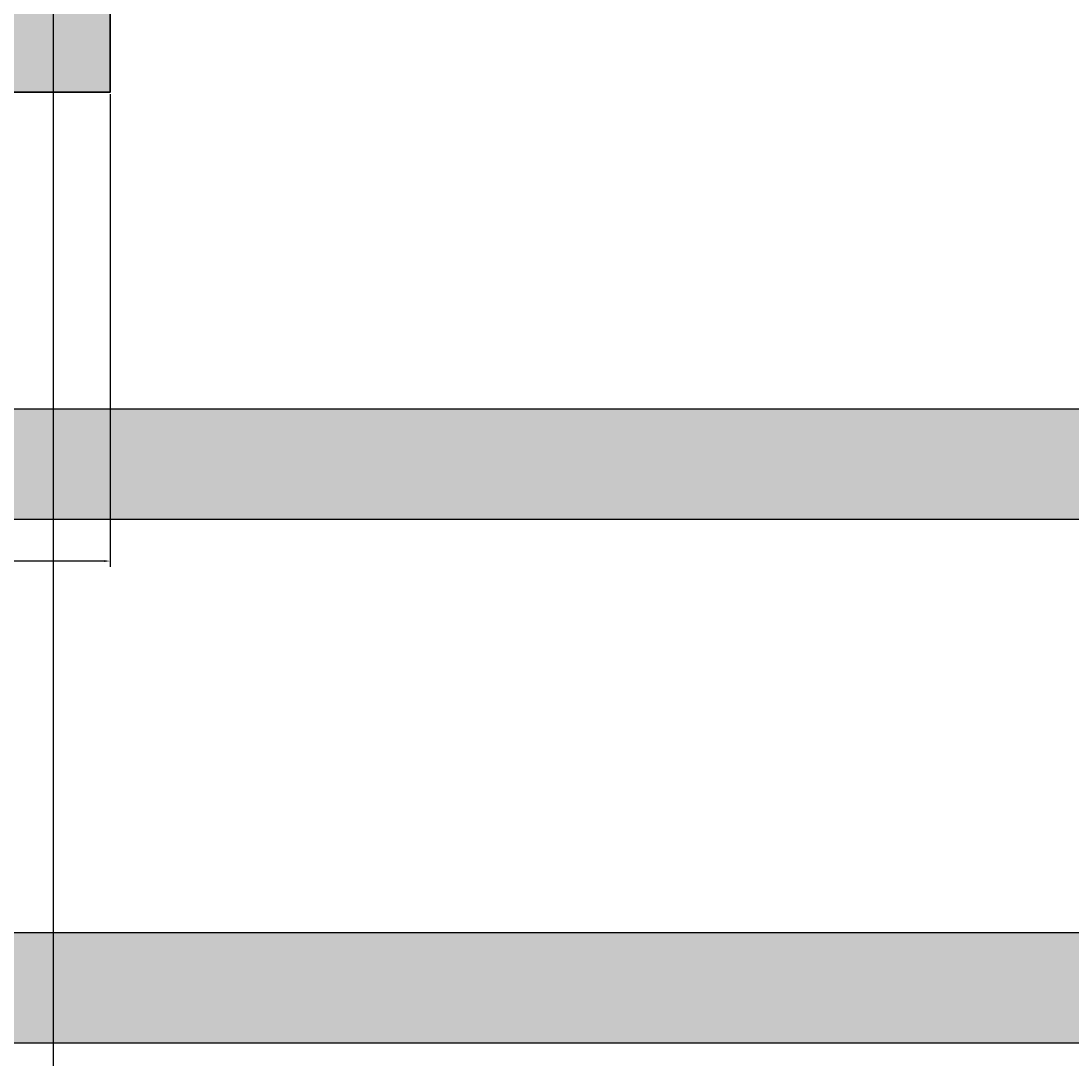
# Model space of a CAD drawing. Units: millimetres. Extents: x -11 to 280, y -4 to 208.
# Tile 4 of 55: x 28 to 61, y 54 to 87. Entities that reach past the tile are written whole.
import ezdxf

# ---------------------------------------------------------------- set-up
doc = ezdxf.new("R2010")
doc.units = ezdxf.units.MM
for name, color, linetype, lineweight in [('M-DIMS', 2, 'Continuous', 18), ('M-HYDR-EQPM', 7, 'Continuous', 35), ('M-HYDR-EQPM-PATT', 252, 'Continuous', 13), ('M-HYDR-RETN', 7, 'Continuous', 25)]:
    doc.layers.add(name, color=color, linetype=linetype, lineweight=lineweight)
doc.layers.add('M-HYDR-RETN-PATT', color=114, linetype='Continuous', lineweight=13, true_color=0x139b48)
doc.styles.get("Standard").update_dxf_attribs({"font": 'arial.ttf'})
doc.dimstyles.get("Standard").update_dxf_attribs({"dimtxt": 0.18, "dimasz": 0.18, "dimexe": 0.18, "dimexo": 0.0625, "dimgap": 0.09, "dimtad": 0, "dimtih": 1, "dimtoh": 1, "dimdec": 4, "dimzin": 0, "dimdsep": 46, "dimtxsty": 'Standard', "dimcen": 0.09, "dimadec": 0, "dimazin": 0, "dimtfac": 1, "dimtdec": 4, "dimtofl": 0, "dimtmove": 0, "dimatfit": 3, "dimfxl": 1, "dimtolj": 1, "dimtzin": 0, "dimarcsym": 0})

# ---------------------------------------------------------------- blocks, each defined once
blk = doc.blocks.new('*D4')
at = {"layer": 'Defpoints', "color": 0, "transparency": 16777216}
for p in [(4.763, 84.426), (266.035, 51.733), (266.035, -3.415)]:
    blk.add_point(p, dxfattribs=at)
at = {"layer": 'M-DIMS', "color": 0, "lineweight": -2, "transparency": 16777216}
for p, q in [((4.763, 84.364), (4.763, -3.595)), ((266.035, 51.67), (266.035, -3.595)), ((4.943, -3.415), (134.934, -3.415)), ((265.855, -3.415), (135.864, -3.415))]:
    blk.add_line(p, q, dxfattribs=at)
at = {"layer": 'M-DIMS', "color": 0, "transparency": 16777216}
for points in [[(4.943, -3.385), (4.943, -3.445), (4.763, -3.415)], [(265.855, -3.385), (265.855, -3.445), (266.035, -3.415)]]:
    blk.add_solid(points, dxfattribs=at)
at = {"layer": 'M-DIMS', "color": 0, "transparency": 16777216, "insert": (135.399, -3.415), "char_height": 0.18, "attachment_point": 5}
blk.add_mtext('\\A1;261.27', dxfattribs=at)
blk = doc.blocks.new('*D5')
at = {"layer": 'Defpoints', "color": 0, "transparency": 16777216}
for p in [(24.759, 192.645), (-10.087, 11.435), (261.686, 11.435)]:
    blk.add_point(p, dxfattribs=at)
at = {"layer": 'M-DIMS', "color": 0, "lineweight": -2, "transparency": 16777216}
for p, q in [((24.696, 192.645), (-10.267, 192.645)), ((-10.087, 192.465), (-10.087, 102.222)), ((-10.087, 11.615), (-10.087, 101.858)), ((261.624, 11.435), (-10.267, 11.435))]:
    blk.add_line(p, q, dxfattribs=at)
at = {"layer": 'M-DIMS', "color": 0, "transparency": 16777216}
for points in [[(-10.117, 192.465), (-10.057, 192.465), (-10.087, 192.645)], [(-10.117, 11.615), (-10.057, 11.615), (-10.087, 11.435)]]:
    blk.add_solid(points, dxfattribs=at)
at = {"layer": 'M-DIMS', "color": 0, "transparency": 16777216, "insert": (-10.087, 102.04), "char_height": 0.18, "attachment_point": 5}
blk.add_mtext('\\A1;181.2', dxfattribs=at)
blk = doc.blocks.new('*D23')
at = {"layer": 'Defpoints', "color": 0, "transparency": 16777216}
for p in [(29.201, 153.977), (66.388, 153.977), (66.388, -3.415)]:
    blk.add_point(p, dxfattribs=at)
at = {"layer": 'M-DIMS', "color": 0, "lineweight": -2, "transparency": 16777216}
for p, q in [((29.201, 153.914), (29.201, -3.595)), ((66.388, 153.914), (66.388, -3.595)), ((29.381, -3.415), (47.331, -3.415)), ((66.208, -3.415), (48.258, -3.415))]:
    blk.add_line(p, q, dxfattribs=at)
at = {"layer": 'M-DIMS', "color": 0, "transparency": 16777216}
for points in [[(29.381, -3.385), (29.381, -3.445), (29.201, -3.415)], [(66.208, -3.385), (66.208, -3.445), (66.388, -3.415)]]:
    blk.add_solid(points, dxfattribs=at)
at = {"layer": 'M-DIMS', "color": 0, "transparency": 16777216, "insert": (47.795, -3.415), "char_height": 0.18, "attachment_point": 5}
blk.add_mtext('\\A1;37.186', dxfattribs=at)
blk = doc.blocks.new('*D27')
at = {"layer": 'Defpoints', "color": 0, "transparency": 16777216}
for p in [(4.763, 84.426), (31.006, 84.426), (4.763, 69.576)]:
    blk.add_point(p, dxfattribs=at)
at = {"layer": 'M-DIMS', "color": 0, "lineweight": -2, "transparency": 16777216}
for p, q in [((4.763, 84.364), (4.763, 69.396)), ((31.006, 84.364), (31.006, 69.396)), ((4.943, 69.576), (17.49, 69.576)), ((30.826, 69.576), (18.28, 69.576))]:
    blk.add_line(p, q, dxfattribs=at)
at = {"layer": 'M-DIMS', "color": 0, "transparency": 16777216}
for points in [[(4.943, 69.606), (4.943, 69.546), (4.763, 69.576)], [(30.826, 69.606), (30.826, 69.546), (31.006, 69.576)]]:
    blk.add_solid(points, dxfattribs=at)
at = {"layer": 'M-DIMS', "color": 0, "transparency": 16777216, "insert": (17.885, 69.576), "char_height": 0.18, "attachment_point": 5}
blk.add_mtext('\\A1;26.24', dxfattribs=at)

msp = doc.modelspace()

# ---------------------------------------------------------------- hatches: boundary and pattern name
at = {"layer": 'M-HYDR-EQPM-PATT'}
h = msp.add_hatch(color=256, dxfattribs=at)
h.set_gradient(color1=(69, 84, 165), color2=(0, 0, 255), tint=1)
h.paths.add_polyline_path([(31.0059, 84.4261), (31.0059, 98.0213), (4.7635, 98.0213), (4.7635, 84.4261)])
at = {"layer": 'M-HYDR-RETN-PATT'}
h = msp.add_hatch(color=256, dxfattribs=at)
h.set_gradient(color1=(19, 155, 72), color2=(19, 155, 72), tint=1)
h.paths.add_polyline_path([(17.9701, 159.0814), (29.2015, 159.0814), (29.2015, 162.5814), (14.4701, 162.5814), (14.4701, 98.0213), (17.9701, 98.0213)])
h.paths.add_polyline_path([(17.9701, 84.4261), (14.4701, 84.4261), (14.4701, 54.3099), (156.2446, 54.3099), (156.2446, 57.8099), (17.9701, 57.8099)])
h.paths.add_polyline_path([(120.5137, 74.3991), (17.9701, 74.3991), (17.9701, 70.8991), (120.5137, 70.8991)], flags=17)
h.paths.add_polyline_path([(184.7092, 75.04, 0.4142136), (179.7092, 80.04), (156.2446, 80.04), (156.2446, 57.8099), (156.2446, 54.3099), (156.2446, 43.5991), (159.7446, 43.5991), (159.7446, 57.8099), (159.7446, 76.54), (176.2092, 76.54, -0.4142136), (181.2092, 71.54), (181.2092, 57.8099), (159.7446, 57.8099), (159.7446, 54.3099), (184.7092, 54.3099)])

# ---------------------------------------------------------------- linework, layer by layer
at = {"layer": 'M-HYDR-EQPM'}
msp.add_lwpolyline([(4.7635, 98.0213), (31.0059, 98.0213), (31.0059, 84.4261), (4.7635, 84.4261)], close=True, dxfattribs=at)
at = {"layer": 'M-HYDR-RETN'}
for points in [[(14.4701, 84.4261), (14.4701, 54.3099), (156.2446, 54.3099)], [(17.9701, 84.4261), (17.9701, 57.8099), (156.2446, 57.8099)], [(17.9701, 74.3991), (120.5137, 74.3991)], [(17.9701, 70.8991), (120.5137, 70.8991)]]:
    msp.add_lwpolyline(points, dxfattribs=at)

# ---------------------------------------------------------------- dimensions: what is measured, and where the dimension line sits
at = {"layer": 'M-DIMS'}
for base, p1, p2, angle, override, picture, middle in [((-10.0865, 11.4346), (24.7588, 192.645), (261.6863, 11.4346), 90, {"dimdec": 1, "dimlfac": 1, "dimrnd": 0, "dimzin": 0, "dimdsep": 46, "dimlunit": 2}, '*D5', (-10.0865, 102.0398)), ((4.7635, 69.5761), (31.0059, 84.4261), (4.7635, 84.4261), 180, {"dimdec": 2, "dimlfac": 1, "dimrnd": 0, "dimzin": 0, "dimdsep": 46, "dimlunit": 2}, '*D27', (17.8847, 69.5761))]:
    dim = msp.add_linear_dim(base=base, p1=p1, p2=p2, angle=angle, dimstyle='Standard', override=override, dxfattribs=at)
    dim.commit()
    dim.dimension.update_dxf_attribs({"geometry": picture, "text_midpoint": middle})
for base, p1, p2, override, picture, middle in [((66.3875, -3.4154), (29.2015, 153.9768), (66.3875, 153.9768), {"dimdec": 3, "dimlfac": 1, "dimrnd": 0, "dimzin": 0, "dimdsep": 46, "dimlunit": 2}, '*D23', (47.7945, -3.4154)), ((266.0352, -3.4154), (4.7635, 84.4261), (266.0352, 51.7328), {"dimdec": 2, "dimlfac": 1, "dimrnd": 0, "dimzin": 0, "dimdsep": 46, "dimlunit": 2}, '*D4', (135.3993, -3.4154))]:
    dim = msp.add_linear_dim(base=base, p1=p1, p2=p2, dimstyle='Standard', override=override, dxfattribs=at)
    dim.commit()
    dim.dimension.update_dxf_attribs({"geometry": picture, "text_midpoint": middle})

doc.saveas('drawing.dxf')
